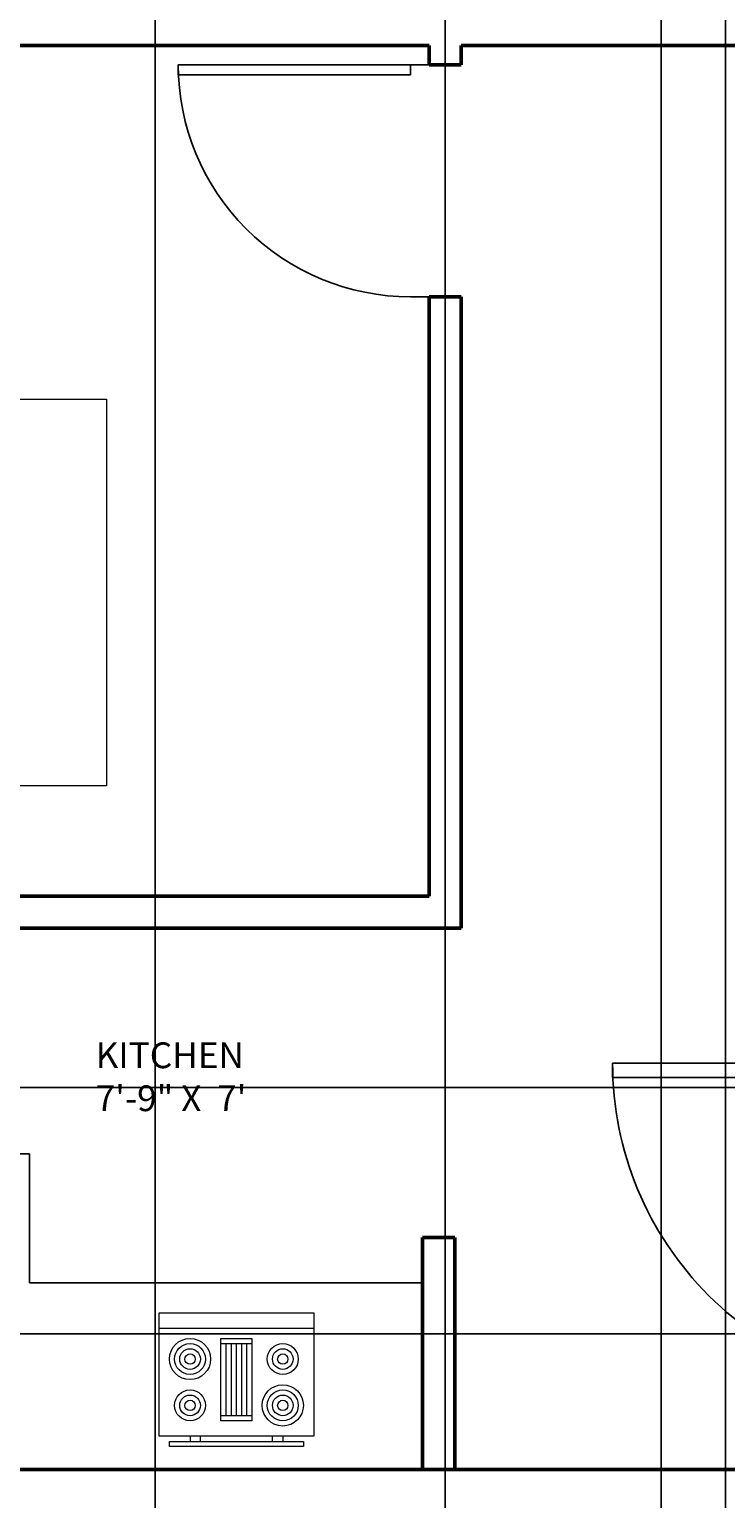
# Model space of a CAD drawing. Units: inches. Extents: x 3506 to 3958, y 1553 to 2506.
# Tile 4 of 16: x 3631 to 3739, y 1775 to 2003. Entities that reach past the tile are written whole.
import ezdxf

# ---------------------------------------------------------------- set-up
doc = ezdxf.new("R2010")
doc.units = ezdxf.units.IN
doc.header["$MEASUREMENT"] = 0
for name, color, linetype, lineweight in [('A-ANNO-DIMS', 2, 'Continuous', 18), ('A-AREA-IDEN', 7, 'Continuous', 18), ('A-FLOR-CASE', 7, 'Continuous', 25), ('A-WALL', 7, 'Continuous', 50), ('doors', 40, 'Continuous', 25), ('furniture', 120, 'Continuous', 18), ('kitchen', 181, 'Continuous', 18)]:
    doc.layers.add(name, color=color, linetype=linetype, lineweight=lineweight)
doc.layers.add('A-WALL-PATT', color=251, linetype='Continuous', lineweight=13, true_color=0x636466)
doc.styles.get("Standard").update_dxf_attribs({"font": 'arial.ttf'})
doc.dimstyles.get("Standard").update_dxf_attribs({"dimtxt": 1.18, "dimasz": 0.68, "dimexe": 0.18, "dimexo": 0.0625, "dimgap": 0.09, "dimtad": 0, "dimtih": 1, "dimtoh": 1, "dimdec": 1, "dimzin": 0, "dimdsep": 46, "dimlunit": 3, "dimtxsty": 'Standard', "dimcen": 0.09, "dimadec": 0, "dimazin": 0, "dimtfac": 1, "dimtdec": 1, "dimtofl": 0, "dimtmove": 0, "dimatfit": 3, "dimfxl": 1, "dimtolj": 1, "dimtzin": 0, "dimarcsym": 0})

# ---------------------------------------------------------------- blocks, each defined once
blk = doc.blocks.new('*U11')
for p, q in [((0, 0), (0, 6)), ((40, 0), (40, 6))]:
    blk.add_line(p, q)
blk.add_lwpolyline([(0, 0), (0, -40), (1.75, -40), (1.75, 0)], close=True)
blk.add_arc((0, 0), 40, 270, 360)
blk = doc.blocks.new('Bed - Queen')
for p, q in [((0, -80.00003), (0, 0)), ((0, 0), (59.99999, 0)), ((59.99999, 0), (59.99999, -80.00003)), ((7.99999, -1.2), (28.79998, -1.2)), ((7.99999, -14.4), (7.99999, -1.2)), ((28.79998, -1.2), (28.79998, -14.4)), ((31.19999, -1.2), (51.99999, -1.2)), ((31.19999, -14.4), (31.19999, -1.2)), ((51.99999, -1.2), (51.99999, -16.4)), ((0, -14.4), (44.8, -14.4)), ((59.99999, -29.6), (44.8, -14.4)), ((44.8, -14.4), (44.8, -29.6)), ((44.8, -16.8), (0, -16.8)), ((51.99999, -16.4), (46.79936, -16.4)), ((44.8, -29.6), (59.99999, -29.6)), ((59.99999, -80.00003), (0, -80.00003))]:
    blk.add_line(p, q)
blk = doc.blocks.new('Range-Oven - 30 in top')
for p, q in [((0, -3), (30, -3)), ((12, -6), (18, -6)), ((13, -20), (13, -6)), ((14, -6), (14, -20)), ((15, -20), (15, -6)), ((16, -6), (16, -20)), ((17, -20), (17, -6)), ((18, -20), (12, -20)), ((6, -24), (6, -25)), ((8, -25), (8, -24)), ((22, -25), (22, -24)), ((24, -24), (24, -25))]:
    blk.add_line(p, q)
for points in [[(0, -24), (0, 0), (30, 0), (30, -24)], [(12, -21), (12, -5), (18, -5), (18, -21)], [(2, -26), (2, -25), (28, -25), (28, -26)]]:
    blk.add_lwpolyline(points, close=True)
for centre, radius in [((6, -9), 4), ((6, -9), 3), ((6, -9), 2), ((6, -9), 1), ((24, -9), 3), ((24, -9), 2), ((24, -9), 1), ((24, -18), 4), ((6, -18), 3), ((6, -18), 2), ((6, -18), 1), ((24, -18), 3), ((24, -18), 2), ((24, -18), 1)]:
    blk.add_circle(centre, radius)
blk = doc.blocks.new('*U12')
for p, q in [((0, 0), (0, 6)), ((40, 0), (40, 6))]:
    blk.add_line(p, q)
blk.add_lwpolyline([(0, 0), (0, -40), (1.75, -40), (1.75, 0)], close=True)
blk.add_arc((0, 0), 40, 270, 0)
blk = doc.blocks.new('*D50')
at = {"layer": 'A-ANNO-DIMS', "color": 0, "lineweight": -2, "transparency": 16777216}
for p, q in [((3608.73, 1606.46), (3608.73, 2505.02)), ((3609.41, 2504.84), (3672.39, 2504.84)), ((3738.05, 2504.84), (3675.07, 2504.84)), ((3738.73, 1606.46), (3738.73, 2505.02))]:
    blk.add_line(p, q, dxfattribs=at)
at = {"layer": 'A-ANNO-DIMS', "color": 0, "transparency": 16777216}
for points in [[(3609.41, 2504.96), (3609.41, 2504.73), (3608.73, 2504.84)], [(3738.05, 2504.96), (3738.05, 2504.73), (3738.73, 2504.84)]]:
    blk.add_solid(points, dxfattribs=at)
at = {"layer": 'Defpoints', "color": 0, "transparency": 16777216}
for p in [(3738.73, 2504.84), (3608.73, 1606.39), (3738.73, 1606.39)]:
    blk.add_point(p, dxfattribs=at)
at = {"layer": 'A-ANNO-DIMS', "color": 0, "transparency": 16777216, "insert": (3673.73, 2504.84), "char_height": 1.18, "attachment_point": 5}
blk.add_mtext('\\A1;130', dxfattribs=at)
blk = doc.blocks.new('*D59')
at = {"layer": 'A-ANNO-DIMS', "color": 0, "lineweight": -2, "transparency": 16777216}
for p, q in [((3728.73, 1689.46), (3728.73, 2505.02)), ((3729.41, 2504.84), (3732.85, 2504.84)), ((3738.05, 2504.84), (3734.61, 2504.84)), ((3738.73, 1689.46), (3738.73, 2505.02))]:
    blk.add_line(p, q, dxfattribs=at)
at = {"layer": 'A-ANNO-DIMS', "color": 0, "transparency": 16777216}
for points in [[(3729.41, 2504.96), (3729.41, 2504.73), (3728.73, 2504.84)], [(3738.05, 2504.96), (3738.05, 2504.73), (3738.73, 2504.84)]]:
    blk.add_solid(points, dxfattribs=at)
at = {"layer": 'Defpoints', "color": 0, "transparency": 16777216}
for p in [(3738.73, 2504.84), (3728.73, 1689.39), (3738.73, 1689.39)]:
    blk.add_point(p, dxfattribs=at)
at = {"layer": 'A-ANNO-DIMS', "color": 0, "transparency": 16777216, "insert": (3733.73, 2504.84), "char_height": 1.18, "attachment_point": 5}
blk.add_mtext('\\A1;10', dxfattribs=at)
blk = doc.blocks.new('*D62')
at = {"layer": 'A-ANNO-DIMS', "color": 0, "lineweight": -2, "transparency": 16777216}
for p, q in [((3860.67, 1838.71), (3508.1, 1838.71)), ((3508.28, 1838.03), (3508.28, 1820.28)), ((3508.28, 1801.14), (3508.28, 1818.89)), ((3860.67, 1800.46), (3508.1, 1800.46))]:
    blk.add_line(p, q, dxfattribs=at)
at = {"layer": 'A-ANNO-DIMS', "color": 0, "transparency": 16777216}
for points in [[(3508.17, 1838.03), (3508.39, 1838.03), (3508.28, 1838.71)], [(3508.17, 1801.14), (3508.39, 1801.14), (3508.28, 1800.46)]]:
    blk.add_solid(points, dxfattribs=at)
at = {"layer": 'Defpoints', "color": 0, "transparency": 16777216}
for p in [(3860.73, 1838.71), (3508.28, 1800.46), (3860.73, 1800.46)]:
    blk.add_point(p, dxfattribs=at)
at = {"layer": 'A-ANNO-DIMS', "color": 0, "transparency": 16777216, "insert": (3508.28, 1819.59), "char_height": 1.18, "attachment_point": 5}
blk.add_mtext('\\A1;38.246', dxfattribs=at)
blk = doc.blocks.new('*D63')
at = {"layer": 'A-ANNO-DIMS', "color": 0, "lineweight": -2, "transparency": 16777216}
for p, q in [((3869.67, 1800.46), (3508.1, 1800.46)), ((3508.28, 1799.78), (3508.28, 1786.12)), ((3508.28, 1771.07), (3508.28, 1784.74)), ((3869.67, 1770.39), (3508.1, 1770.39))]:
    blk.add_line(p, q, dxfattribs=at)
at = {"layer": 'A-ANNO-DIMS', "color": 0, "transparency": 16777216}
for points in [[(3508.17, 1799.78), (3508.39, 1799.78), (3508.28, 1800.46)], [(3508.17, 1771.07), (3508.39, 1771.07), (3508.28, 1770.39)]]:
    blk.add_solid(points, dxfattribs=at)
at = {"layer": 'Defpoints', "color": 0, "transparency": 16777216}
for p in [(3869.73, 1800.46), (3508.28, 1770.39), (3869.73, 1770.39)]:
    blk.add_point(p, dxfattribs=at)
at = {"layer": 'A-ANNO-DIMS', "color": 0, "transparency": 16777216, "insert": (3508.28, 1785.43), "char_height": 1.18, "attachment_point": 5}
blk.add_mtext('\\A1;30.07', dxfattribs=at)
blk = doc.blocks.new('*D66')
at = {"layer": 'A-ANNO-DIMS', "color": 0, "lineweight": -2, "transparency": 16777216}
for p, q in [((3650.23, 2221.36), (3650.23, 1553.76)), ((3695.23, 2221.36), (3695.23, 1553.76)), ((3650.91, 1553.94), (3671.77, 1553.94)), ((3694.55, 1553.94), (3673.69, 1553.94))]:
    blk.add_line(p, q, dxfattribs=at)
at = {"layer": 'A-ANNO-DIMS', "color": 0, "transparency": 16777216}
for points in [[(3650.91, 1554.06), (3650.91, 1553.83), (3650.23, 1553.94)], [(3694.55, 1554.06), (3694.55, 1553.83), (3695.23, 1553.94)]]:
    blk.add_solid(points, dxfattribs=at)
at = {"layer": 'Defpoints', "color": 0, "transparency": 16777216}
for p in [(3650.23, 2221.43), (3695.23, 2221.43), (3695.23, 1553.94)]:
    blk.add_point(p, dxfattribs=at)
at = {"layer": 'A-ANNO-DIMS', "color": 0, "transparency": 16777216, "insert": (3672.73, 1553.94), "char_height": 1.18, "attachment_point": 5}
blk.add_mtext('\\A1;45', dxfattribs=at)

msp = doc.modelspace()

# ---------------------------------------------------------------- hatches: boundary and pattern name
at = {"layer": 'A-WALL-PATT'}
h = msp.add_hatch(dxfattribs=at)
h.set_pattern_fill('ANSI31', color=256)
h.paths.add_polyline_path([(3911.7302, 2461.3942), (3551.7302, 2461.3942), (3551.7302, 2152.516), (3560.7302, 2152.516), (3560.7302, 2116.516), (3551.7302, 2116.516), (3551.7302, 1920.5711), (3556.2302, 1920.5711), (3560.7302, 1920.5711), (3560.7302, 2000.3942), (3692.7302, 2000.3942), (3692.7302, 1997.3942), (3697.7302, 1997.3942), (3697.7302, 2000.3942), (3771.7302, 2000.3942), (3771.7302, 1997.3942), (3776.7302, 1997.3942), (3776.7302, 1997.7206), (3778.5802, 1997.7206), (3807.5802, 1997.7206), (3807.5802, 1996.4519), (3778.5802, 1996.4519), (3778.5802, 1997.7206), (3776.7302, 1997.7206), (3776.7302, 1997.3942), (3771.7302, 1997.3942), (3771.7302, 2000.3942), (3697.7302, 2000.3942), (3697.7302, 1997.3942), (3692.7302, 1997.3942), (3689.8302, 1997.3942), (3689.8302, 1995.8192), (3653.8302, 1995.8192), (3653.8302, 1997.3942), (3689.8302, 1997.3942), (3692.7302, 1997.3942), (3692.7302, 2000.3942), (3560.7302, 2000.3942), (3560.7302, 1920.5711), (3551.7302, 1920.5711), (3551.7302, 1884.5711), (3551.7302, 1597.3942), (3911.7302, 1597.3942)], flags=17)
h.paths.add_polyline_path([(3596.7302, 2005.3942), (3596.7302, 2057.3035, -0.38730371), (3569.1778, 2085), (3569.15, 2085), (3569.15, 2086.2688), (3598.15, 2086.2688), (3598.15, 2085), (3569.1778, 2085, 0.38730371), (3596.7302, 2057.3035), (3596.7302, 2057.3942), (3601.7302, 2057.3942), (3601.7302, 2055.3942), (3630.7302, 2055.3942), (3630.7302, 2034.3942), (3694.7302, 2034.3942), (3694.7302, 2053.3942), (3699.7302, 2053.3942), (3699.7302, 2005.3942), (3860.7302, 2005.3942), (3860.7302, 2173.3942), (3771.7302, 2173.3942), (3771.7302, 2194.3942), (3776.7302, 2194.3942), (3776.7302, 2178.3942), (3860.7302, 2178.3942), (3860.7302, 2231.3942), (3601.7302, 2231.3942), (3601.7302, 2241.426), (3596.7302, 2241.426), (3596.7302, 2231.3942), (3560.7302, 2231.3942), (3560.7302, 2315.3942), (3596.7302, 2315.3942), (3596.7302, 2312.3942), (3601.7302, 2312.3942), (3601.7302, 2315.3942), (3697.7302, 2315.3942), (3697.7302, 2413.3942), (3692.7302, 2413.3942), (3692.7302, 2320.3942), (3560.7302, 2320.3942), (3560.7302, 2452.3942), (3692.7302, 2452.3942), (3692.7302, 2449.3942), (3697.7302, 2449.3942), (3697.7302, 2452.3942), (3771.7302, 2452.3942), (3771.7302, 2449.3942), (3776.7302, 2449.3942), (3776.7302, 2452.3942), (3860.7302, 2452.3942), (3860.7302, 2437.2075), (3865.2302, 2437.2075), (3865.2302, 2413.2075), (3860.7302, 2413.2075), (3860.7302, 2367.6976), (3865.2302, 2367.6976), (3869.7302, 2367.6976), (3869.7302, 2319.6976), (3860.7302, 2319.6976), (3860.7302, 2211.6248), (3869.7302, 2211.6248), (3869.7302, 2187.6248), (3860.7302, 2187.6248), (3860.7302, 2138.4346), (3865.2302, 2138.4346), (3869.7302, 2138.4346), (3869.7302, 2090.4346), (3860.7302, 2090.4346), (3860.7302, 1985.8449), (3869.7302, 1985.8449), (3869.7302, 1961.8449), (3860.7302, 1961.8449), (3860.7302, 1897.0756), (3865.2302, 1897.0756), (3869.7302, 1897.0756), (3869.7302, 1849.0756), (3860.7302, 1849.0756), (3860.7302, 1847.8112), (3860.7302, 1779.3942), (3596.7302, 1779.3942), (3596.7302, 1831.3942), (3601.7302, 1831.3942), (3601.7302, 1828.3942), (3630.7302, 1828.3942), (3630.7302, 1808.3942), (3691.7302, 1808.3942), (3691.7302, 1815.3942), (3696.7302, 1815.3942), (3696.7302, 1779.3942), (3860.7302, 1779.3942), (3860.7302, 1947.3942), (3771.7302, 1947.3942), (3771.7302, 1968.3942), (3776.7302, 1968.3942), (3776.7302, 1952.3942), (3860.7302, 1952.3942), (3860.7302, 2005.3942)], flags=0)
h.paths.add_polyline_path([(3596.7302, 2038.8546), (3601.7302, 2038.8546), (3601.7302, 2014.8546), (3596.7302, 2014.8546)], flags=0)
h.paths.add_polyline_path([(3564.1688, 2107), (3564.1688, 2167), (3644.1688, 2167), (3644.1688, 2107)], flags=0)
h.paths.add_polyline_path([(3607.0972, 2052.0208), (3620.8472, 2052.0208, -0.41421356), (3621.9931, 2050.875), (3621.9931, 2025.6667, -0.41421356), (3620.8472, 2024.5208), (3607.0972, 2024.5208, -0.41421356), (3605.9514, 2025.6667), (3605.9514, 2050.875, -0.41421356)], flags=0)
h.paths.add_polyline_path([(3578.5688, 2115), (3565.3688, 2115), (3565.3688, 2135.8), (3578.5688, 2135.8), (3578.5688, 2138.2), (3565.3688, 2138.2), (3565.3688, 2159), (3580.5688, 2159), (3580.5688, 2153.8), (3593.7688, 2167), (3593.7688, 2151.8), (3578.5688, 2151.8)], flags=0)
h.paths.add_polyline_path([(3610.9167, 2050.875), (3620.0833, 2050.875, -0.41421356), (3620.8472, 2050.1111), (3620.8472, 2039.6076, -0.41421356), (3620.0833, 2038.8438), (3610.9167, 2038.8438, -0.41421356), (3610.1528, 2039.6076), (3610.1528, 2050.1111, -0.41421356)], flags=0)
h.paths.add_polyline_path([(3610.9167, 2037.6979), (3620.0833, 2037.6979, -0.41421356), (3620.8472, 2036.934), (3620.8472, 2026.4306, -0.41421356), (3620.0833, 2025.6667), (3610.9167, 2025.6667, -0.41421356), (3610.1528, 2026.4306), (3610.1528, 2036.934, -0.41421356)], flags=0)
h.paths.add_polyline_path([(3616.2639, 2044.7639, -1), (3614.7361, 2044.7639, -1)], flags=0)
h.paths.add_polyline_path([(3615.8819, 2044.7639, -1), (3615.1181, 2044.7639, -1)], flags=0)
h.paths.add_polyline_path([(3616.2639, 2031.7778, -1), (3614.7361, 2031.7778, -1)], flags=0)
h.paths.add_polyline_path([(3615.8819, 2031.7778, -1), (3615.1181, 2031.7778, -1)], flags=0)
h.paths.add_polyline_path([(3609.7539, 2021.7868), (3626.9586, 2021.7868), (3626.9586, 2008.8833), (3609.7539, 2008.8833)], flags=0)
h.paths.add_polyline_path([(3610.4708, 2021.07), (3621.2237, 2021.07), (3621.2237, 2009.6002), (3610.4708, 2009.6002)], flags=0)
h.paths.add_polyline_path([(3611.5461, 2019.9947), (3620.1484, 2019.9947), (3620.1484, 2010.6755), (3611.5461, 2010.6755)], flags=0)
h.paths.add_polyline_path([(3621.9405, 2021.07), (3626.2417, 2021.07), (3626.2417, 2009.6002), (3621.9405, 2009.6002)], flags=0)
h.paths.add_polyline_path([(3622.6574, 2020.3531), (3625.5248, 2020.3531), (3625.5248, 2017.4857), (3622.6574, 2017.4857)], flags=0)
h.paths.add_polyline_path([(3622.6574, 2016.7688), (3625.5248, 2016.7688), (3625.5248, 2010.317), (3622.6574, 2010.317)], flags=0)
h.paths.add_polyline_path([(3624.808, 2016.0519), (3624.808, 2013.9013), (3624.0911, 2013.9013), (3624.0911, 2013.1845), (3623.3743, 2013.1845), (3623.3743, 2013.9013), (3623.3743, 2016.0519)], flags=0)
h.paths.add_polyline_path([(3623.0158, 2012.8261), (3625.1664, 2012.8261), (3625.1664, 2012.1092), (3623.0158, 2012.1092)], flags=0)
h.paths.add_polyline_path([(3623.0158, 2011.7508), (3625.1664, 2011.7508), (3625.1664, 2011.0339), (3623.0158, 2011.0339)], flags=0)
h.paths.add_polyline_path([(3650.0591, 2031.8202), (3674.0368, 2031.8202), (3674.0368, 2012.638), (3669.2413, 2012.638), (3669.2413, 2011.8388), (3672.4383, 2011.8388), (3672.4383, 2011.0395), (3651.6576, 2011.0395), (3651.6576, 2011.8388), (3654.8546, 2011.8388), (3654.8546, 2012.638), (3650.0591, 2012.638)], flags=0)
h.paths.add_polyline_path([(3658.0517, 2024.6269, -1), (3651.6576, 2024.6269, -1)], flags=0)
h.paths.add_polyline_path([(3657.2524, 2024.6269, -1), (3652.4569, 2024.6269, -1)], flags=0)
h.paths.add_polyline_path([(3656.4532, 2024.6269, -1), (3653.2561, 2024.6269, -1)], flags=0)
h.paths.add_polyline_path([(3655.6539, 2024.6269, -1), (3654.0554, 2024.6269, -1)], flags=0)
h.paths.add_polyline_path([(3657.2524, 2017.4336, -1), (3652.4569, 2017.4336, -1)], flags=0)
h.paths.add_polyline_path([(3656.4532, 2017.4336, -1), (3653.2561, 2017.4336, -1)], flags=0)
h.paths.add_polyline_path([(3655.6539, 2017.4336, -1), (3654.0554, 2017.4336, -1)], flags=0)
h.paths.add_polyline_path([(3659.6502, 2027.8239), (3664.4457, 2027.8239), (3664.4457, 2015.0358), (3659.6502, 2015.0358)], flags=0)
h.paths.add_polyline_path([(3663.6465, 2027.0247), (3663.6465, 2015.8351), (3660.4494, 2015.8351), (3660.4494, 2027.0247)], flags=0)
h.paths.add_polyline_path([(3562.6688, 1945.5), (3642.6688, 1945.5), (3642.6688, 1885.5), (3562.6688, 1885.5)], flags=0)
h.paths.add_polyline_path([(3671.6391, 2024.6269, -1), (3666.8435, 2024.6269, -1)], flags=0)
h.paths.add_polyline_path([(3670.8398, 2024.6269, -1), (3667.6428, 2024.6269, -1)], flags=0)
h.paths.add_polyline_path([(3672.4383, 2017.4336, -1), (3666.0443, 2017.4336, -1)], flags=0)
h.paths.add_polyline_path([(3670.0405, 2024.6269, -1), (3668.442, 2024.6269, -1)], flags=0)
h.paths.add_polyline_path([(3671.6391, 2017.4336, -1), (3666.8435, 2017.4336, -1)], flags=0)
h.paths.add_polyline_path([(3670.8398, 2017.4336, -1), (3667.6428, 2017.4336, -1)], flags=0)
h.paths.add_polyline_path([(3592.2688, 1945.5), (3592.2688, 1930.3), (3577.0688, 1930.3), (3577.0688, 1893.5), (3563.8688, 1893.5), (3563.8688, 1914.3), (3577.0688, 1914.3), (3577.0688, 1916.7), (3563.8688, 1916.7), (3563.8688, 1937.5), (3579.0688, 1937.5), (3579.0688, 1932.3)], flags=0)
h.paths.add_polyline_path([(3670.0405, 2017.4336, -1), (3668.442, 2017.4336, -1)], flags=0)
h.paths.add_polyline_path([(3596.7302, 2283.3942), (3601.7302, 2283.3942), (3601.7302, 2265.426), (3599.2302, 2265.426), (3599.2302, 2241.426), (3596.7302, 2241.426), (3596.7302, 2265.426)], flags=0)
h.paths.add_polyline_path([(3596.7302, 1810.7006), (3601.7302, 1810.7006), (3601.7302, 1786.7006), (3596.7302, 1786.7006)], flags=0)
h.paths.add_polyline_path([(3560.7302, 1770.3942), (3738.7302, 1770.3942), (3738.7302, 1746.3942), (3738.7302, 1722.3942), (3748.7302, 1722.3942), (3748.7302, 1674.3942), (3560.7302, 1674.3942)], flags=0)
h.paths.add_polyline_path([(3728.7302, 1746.3942), (3728.7302, 1756.0642), (3738.7302, 1746.3942), (3728.7302, 1738.1582), (3728.7302, 1698.3942), (3591.2519, 1698.3942), (3591.2519, 1746.3942)], flags=0)
h.paths.add_polyline_path([(3771.7302, 2399.3942), (3771.7302, 2420.3942), (3776.7302, 2420.3942), (3776.7302, 2404.3942), (3776.7302, 2399.3942)], flags=0)
h.paths.add_polyline_path([(3911.7302, 2461.3942), (3551.7302, 2461.3942), (3551.7302, 2152.516), (3560.7302, 2152.516), (3560.7302, 2116.516), (3551.7302, 2116.516), (3551.7302, 1920.5711), (3560.7302, 1920.5711), (3560.7302, 2000.3942), (3692.7302, 2000.3942), (3692.7302, 1997.3942), (3697.7302, 1997.3942), (3697.7302, 2000.3942), (3771.7302, 2000.3942), (3771.7302, 1997.3942), (3776.7302, 1997.3942), (3776.7302, 1997.7206), (3778.5802, 1997.7206), (3807.5802, 1997.7206), (3807.5802, 1996.4519), (3778.5802, 1996.4519), (3778.5802, 1997.7206), (3776.7302, 1997.7206), (3776.7302, 1997.3942), (3771.7302, 1997.3942), (3771.7302, 2000.3942), (3697.7302, 2000.3942), (3697.7302, 1997.3942), (3692.7302, 1997.3942), (3689.8302, 1997.3942), (3689.8302, 1995.8192), (3653.8302, 1995.8192), (3653.8302, 1997.3942), (3689.8302, 1997.3942), (3692.7302, 1997.3942), (3692.7302, 2000.3942), (3560.7302, 2000.3942), (3560.7302, 1920.5711), (3551.7302, 1920.5711), (3551.7302, 1597.3942), (3911.7302, 1597.3942)], flags=17)

# ---------------------------------------------------------------- linework, layer by layer
at = {"layer": 'A-FLOR-CASE'}
for p, q in [((3601.7302, 1828.3942), (3630.7302, 1828.3942)), ((3630.7302, 1808.3942), (3630.7302, 1828.3942)), ((3630.7302, 1808.3942), (3691.7302, 1808.3942))]:
    msp.add_line(p, q, dxfattribs=at)
at = {"layer": 'A-WALL'}
for p, q in [((3560.7302, 2000.3942), (3692.7302, 2000.3942)), ((3692.7302, 2000.3942), (3692.7302, 1997.3942)), ((3692.7302, 1997.3942), (3692.7302, 2000.3942)), ((3697.7302, 1997.3942), (3697.7302, 2000.3942)), ((3697.7302, 2000.3942), (3771.7302, 2000.3942)), ((3692.7302, 1997.3942), (3697.7302, 1997.3942)), ((3692.7302, 1868.3942), (3692.7302, 1961.3942)), ((3692.7302, 1961.3942), (3697.7302, 1961.3942)), ((3697.7302, 1961.3942), (3697.7297, 1961.3942)), ((3697.7302, 1868.3942), (3697.7302, 1961.3942)), ((3697.7302, 1961.3942), (3697.7302, 1961.3939)), ((3697.7302, 1961.3939), (3697.7302, 1961.3942)), ((3560.7302, 1868.3942), (3692.7302, 1868.3942)), ((3697.7302, 1868.3942), (3697.7302, 1863.3942)), ((3601.7302, 1863.3942), (3697.7302, 1863.3942)), ((3691.7302, 1779.3942), (3691.7302, 1815.3942)), ((3691.7302, 1815.3942), (3696.7302, 1815.3942)), ((3696.7302, 1779.3942), (3696.7302, 1815.3942)), ((3560.7302, 1779.3942), (3771.7302, 1779.3942))]:
    msp.add_line(p, q, dxfattribs=at)

# ---------------------------------------------------------------- block references
at = {"layer": 'doors', "rotation": 270}
for name, p, xscale, yscale, zscale in [('*U11', (3689.8302, 1997.3942), 0.9000000000000001, 0.9000000000000001, 0.9000000000000001), ('*U12', (3772.2282, 1842.4626), 1.27563568336709, 1.27563568336709, 1.27563568336709)]:
    msp.add_blockref(name, p, dxfattribs=dict(at, xscale=xscale, yscale=yscale, zscale=zscale))
at = {"layer": 'furniture', "rotation": 90}
msp.add_blockref('Bed - Queen', (3562.6688, 1885.5), dxfattribs=at)
at = {"layer": 'kitchen', "xscale": 0.7992583991282335, "yscale": 0.7992583991282335, "zscale": 0.7992583991282335}
msp.add_blockref('Range-Oven - 30 in top', (3650.8583, 1803.7483), dxfattribs=at)

# ---------------------------------------------------------------- texts
at = {"layer": 'A-AREA-IDEN', "insert": (3641.0073, 1845.6951), "char_height": 4, "attachment_point": 1}
msp.add_mtext_dynamic_manual_height_columns('KITCHEN\\P7\'-9" X  7\'', width=34.025371, gutter_width=1, heights=[0], dxfattribs=at)

# ---------------------------------------------------------------- dimensions: what is measured, and where the dimension line sits
at = {"layer": 'A-ANNO-DIMS'}
for base, p1, p2, picture, middle in [((3738.7302, 2504.8442), (3608.7302, 1606.3942), (3738.7302, 1606.3942), '*D50', (3673.7302, 2504.8442)), ((3738.7302, 2504.8442), (3728.7302, 1689.3942), (3738.7302, 1689.3942), '*D59', (3733.7302, 2504.8442)), ((3695.2302, 1553.9442), (3650.2302, 2221.4254), (3695.2302, 2221.4254), '*D66', (3672.7302, 1553.9442))]:
    dim = msp.add_linear_dim(base=base, p1=p1, p2=p2, dimstyle='Standard', override={"dimdec": 0, "dimlfac": 1, "dimrnd": 0, "dimzin": 0, "dimdsep": 46, "dimlunit": 2}, dxfattribs=at)
    dim.commit()
    dim.dimension.update_dxf_attribs({"geometry": picture, "text_midpoint": middle})
for base, p1, p2, override, picture, middle in [((3508.2802, 1800.4628), (3860.7302, 1838.7087), (3860.7302, 1800.4628), {"dimdec": 3, "dimlfac": 1, "dimrnd": 0, "dimzin": 0, "dimdsep": 46, "dimlunit": 2}, '*D62', (3508.2802, 1819.5857)), ((3508.2802, 1770.3942), (3869.7302, 1800.4628), (3869.7302, 1770.3942), {"dimdec": 2, "dimlfac": 1, "dimrnd": 0, "dimzin": 0, "dimdsep": 46, "dimlunit": 2}, '*D63', (3508.2802, 1785.4285))]:
    dim = msp.add_linear_dim(base=base, p1=p1, p2=p2, angle=90, dimstyle='Standard', override=override, dxfattribs=at)
    dim.commit()
    dim.dimension.update_dxf_attribs({"geometry": picture, "text_midpoint": middle})

doc.saveas('drawing.dxf')
